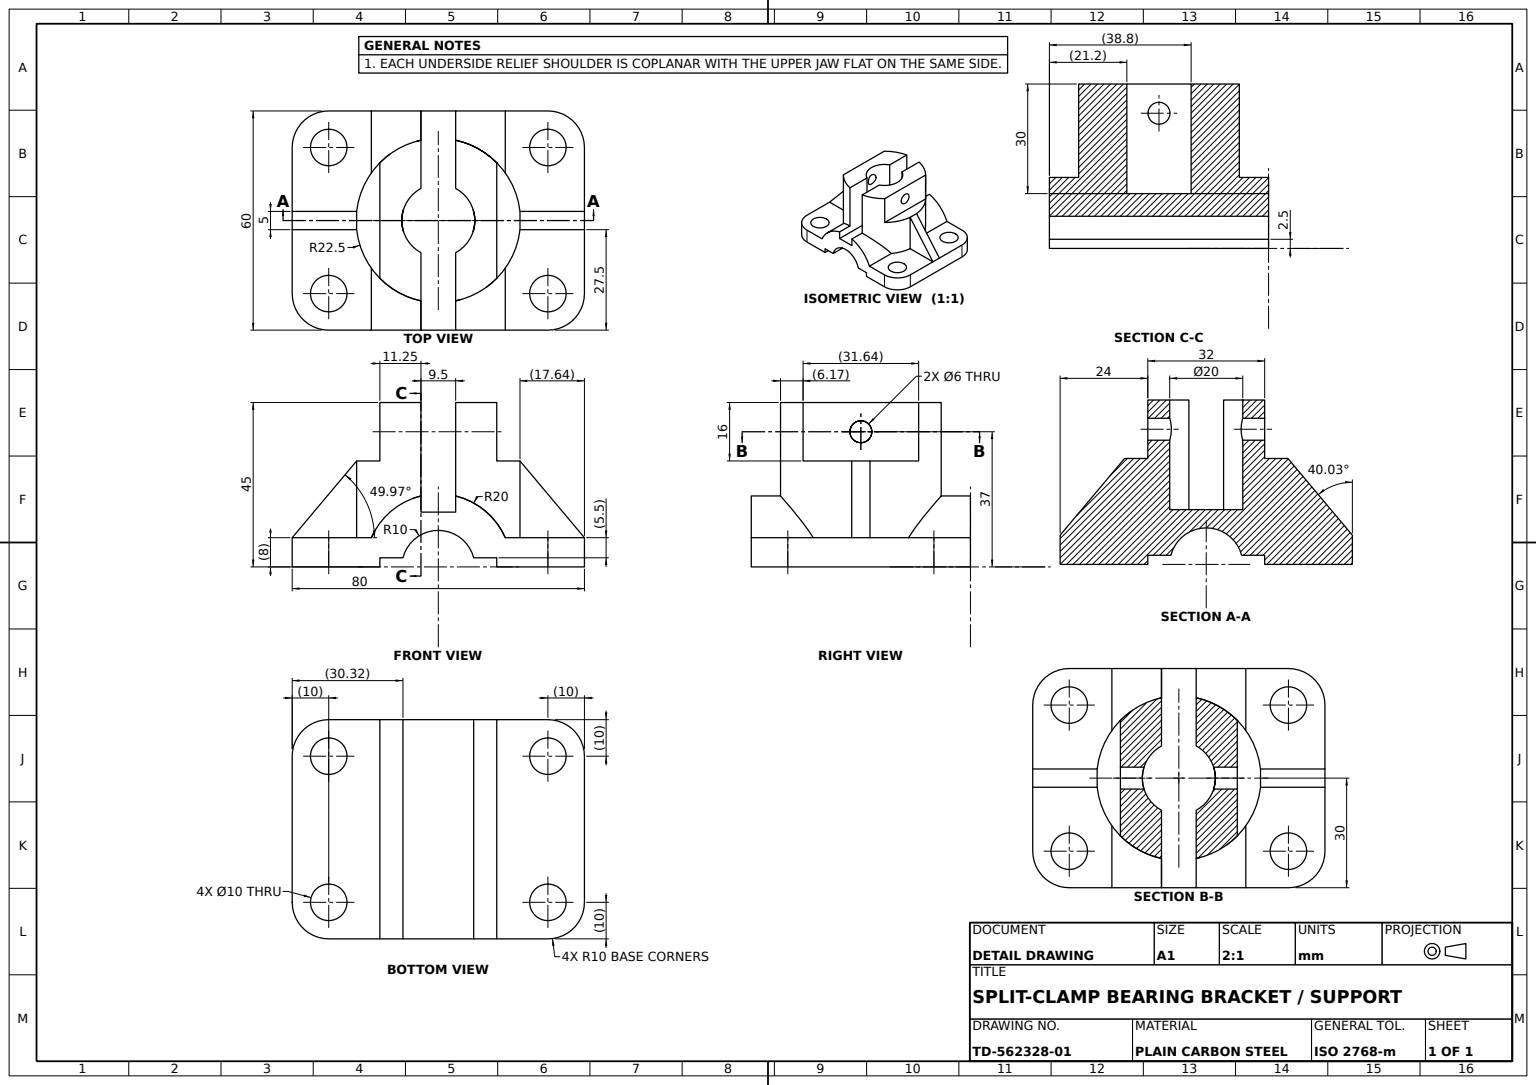
SolidWorks part; units mm, degrees
material "Plain Carbon Steel"
ref_plane "Front Plane" through (0, 0, 0) normal (0, 0, 1) x (1, 0, 0)
ref_plane "Top Plane" through (0, 0, 0) normal (0, 1, 0) x (1, 0, 0)
ref_plane "Right Plane" through (0, 0, 0) normal (1, 0, 0) x (0, 0, -1)
sketch "Base Profile Sketch" plane through (0, 0, 0) normal (0, 0, 1) x (1, 0, 0)
  line L0 (0, 0) -> (0, 8)
  line L1 (0, 8) -> (21.6697, 8)
  line L2 (80, 8) -> (80, 0)
  line L3 (80, 0) -> (56, 0)
  line L4 (56, 0) -> (56, 2.5)
  line L5 (56, 2.5) -> (49.6825, 2.5)
  line L6 (24, 2.5) -> (24, 0)
  line L7 (24, 0) -> (0, 0)
  line L9 (30.3175, 2.5) -> (24, 2.5)
  line L10 (58.3303, 8) -> (80, 8)
  arc A0 (49.6825, 2.5) -> (30.3175, 2.5) centre (40, 0) ccw
  arc A1 (58.3303, 8) -> (21.6697, 8) centre (40, 0) ccw
  dimension "D8" = 40
  dimension "D9" = 20
  dimension "D10" = 30.3175
  dimension "D1" = 8
  dimension "D2" = 32
  dimension "D3" = 24
  dimension "D4" = 80
  dimension "D5" = 2.5
  dimension "D6" = 2.5
  dimension "D7" = 5.5
  dimension "D11" = 28.0128
extrude "Base Body" add sketch "Base Profile Sketch" against normal blind 60
ref_plane "Boss Top Plane" through (0, 45, 0) normal (0, 1, 0) x (1, 0, 0)
sketch "Vertical Boss Sketch" plane through (0, 45, 0) normal (0, 1, 0) x (1, 0, 0)
  circle A0 centre (40, 30) radius 22.5
  dimension "D1" = 45
  dimension "D2" = 40
  dimension "D3" = 30
extrude "Vertical Boss Ø40" add sketch "Vertical Boss Sketch" against normal blind 38
sketch "Base Half Bore Sketch" plane through (0, 0, 0) normal (0, 0, 1) x (1, 0, 0)
  circle A0 centre (40, 0) radius 10
  dimension "D1" = 20
extrude "Base Half Bore Ø20" cut sketch "Base Half Bore Sketch" against normal blind 60
fillet "Base Corner Fillets R10" radius 10 4 edges at (0, 4, -60) (0, 4, 0) (80, 4, -60) (80, 4, 0)
sketch "Mounting Holes Sketch" plane through (0, 8, 0) normal (0, 1, 0) x (1, 0, 0)
  line L0 (70, 60) -> (58.3303, 60) construction
  line L1 (80, 50) -> (80, 10) construction
  line L2 (70, 0) -> (58.3303, 0) construction
  line L3 (21.6697, 0) -> (10, 0) construction
  line L4 (0, 50) -> (0, 10) construction
  line L5 (21.6697, 60) -> (10, 60) construction
  circle A0 centre (70, 50) radius 5
  circle A1 centre (70, 10) radius 5
  circle A2 centre (10, 10) radius 5
  circle A3 centre (10, 50) radius 5
  dimension "D1" = 10
  dimension "D2" = 10
  dimension "D3" = 10
  dimension "D4" = 10
  dimension "D5" = 10
  dimension "D6" = 10
  dimension "D7" = 10
  dimension "D8" = 10
  dimension "D9" = 10
  dimension "D10" = 10
  dimension "D11" = 10
  dimension "D12" = 10
extrude "Mounting Holes 4xØ10" cut sketch "Mounting Holes Sketch" against normal blind 60
sketch "Rib Profile Sketch" plane through (0, 45, 0) normal (0, 1, 0) x (1, 0, 0)
  line L0 (35.25, 38.7999) -> (35.25, 60)
  line L2 (44.75, 0) -> (44.75, 21.2001)
  line L3 (35.25, 0) -> (35.25, 21.2001)
  line L4 (44.75, 38.7999) -> (44.75, 60)
  line L5 (35.25, 60) -> (44.75, 60)
  line L6 (35.25, 0) -> (44.75, 0)
  arc A0 (35.25, 38.7999) -> (35.25, 21.2001) centre (40, 30) ccw
  arc A1 (44.75, 21.2001) -> (44.75, 38.7999) centre (40, 30) ccw
  point P8 (40, 30)
  dimension "D1" = 20
  dimension "D2" = 9.5
  dimension "D3" = 21.2001
  dimension "D4" = 38.7999
  dimension "D5" = 9.5
  dimension "D6" = 60
  dimension "D7" = 38.7999
extrude "Rib Profile Cut" cut sketch "Rib Profile Sketch" against normal blind 30
sketch "Boss Upper Bore Sketch" plane through (0, 45, 0) normal (0, 1, 0) x (1, 0, 0)
  line L0 (44.75, 38.7999) -> (44.75, 51.9929) construction
  line L3 (56, 14.1807) -> (56, 45.8193)
  line L4 (24, 14.1807) -> (24, 45.8193)
  arc A0 (24, 45.8193) -> (24, 14.1807) centre (40, 30) ccw
  arc A2 (56, 45.8193) -> (56, 14.1807) centre (40, 30) cw
  dimension "D1" = 32
  dimension "D2" = 22.5
  dimension "D3" = 22.5
  dimension "D4" = 31.6386
  dimension "D5" = 16
  dimension "D6" = 15.8193
  dimension "D7" = 31.6386
  dimension "D8" = 11.25
  dimension "D9" = 6.1736
extrude "Boss Upper Bore Cut" cut sketch "Boss Upper Bore Sketch" against normal blind 16
sketch "Boss Lower Bore Sketch" plane through (56, 0, 0) normal (1, 0, 0) x (0, 0, -1)
  line L0 (45.8193, 45) -> (14.1807, 45) construction
  circle A0 centre (30, 37) radius 3
  dimension "D1" = 6
  dimension "D2" = 8
  dimension "D3" = 15.8193
extrude "Boss Lower Bore Cut" cut sketch "Boss Lower Bore Sketch" against normal through all
ref_plane "Lug Plane X62" through (62, 0, 0) normal (1, 0, 0) x (0, 0, -1)
sketch "Clamp Lug X62 Sketch" plane through (62, 0, 0) normal (1, 0, 0) x (0, 0, -1)
  line L0 (45.8193, 29) -> (14.1807, 29) construction
  line L1 (27.5, 29) -> (32.5, 29)
  line L2 (27.5, 29) -> (27.5, 8)
  line L3 (27.5, 8) -> (32.5, 8)
  line L4 (32.5, 29) -> (32.5, 8)
  line L5 (50, 8) -> (10, 8) construction
  dimension "D1" = 5
  dimension "D2" = 27.5
extrude "Clamp Lug X62" add sketch "Clamp Lug X62 Sketch" along normal blind 18
sketch "Lug X62 Hole Sketch" plane through (0, 0, -27.5) normal (0, 0, 1) x (1, 0, 0)
  line L0 (62.3607, 29) -> (80, 8)
extrude "Lug X62 Hole Cut" cut sketch "Lug X62 Hole Sketch" against normal blind 18 and the other way through all
ref_plane "Lug Plane X18" through (18, 0, 0) normal (1, 0, 0) x (0, 0, -1)
sketch "Clamp Lug X18 Sketch" plane through (18, 0, 0) normal (1, 0, 0) x (0, 0, -1)
  line L0 (45.8193, 29) -> (14.1807, 29) construction
  line L1 (32.5, 29) -> (27.5, 29)
  line L2 (32.5, 29) -> (32.5, 8)
  line L3 (32.5, 8) -> (27.5, 8)
  line L4 (27.5, 29) -> (27.5, 8)
  line L5 (50, 8) -> (10, 8) construction
  dimension "D1" = 5
  dimension "D2" = 27.5
extrude "Clamp Lug X18" add sketch "Clamp Lug X18 Sketch" against normal blind 18
sketch "Lug X18 Hole Sketch" plane through (0, 0, -32.5) normal (0, 0, -1) x (-1, 0, 0)
  line L0 (-17.6393, 29) -> (0, 8)
extrude "Lug X18 Hole Cut" cut sketch "Lug X18 Hole Sketch" against normal blind 18 and the other way through all
